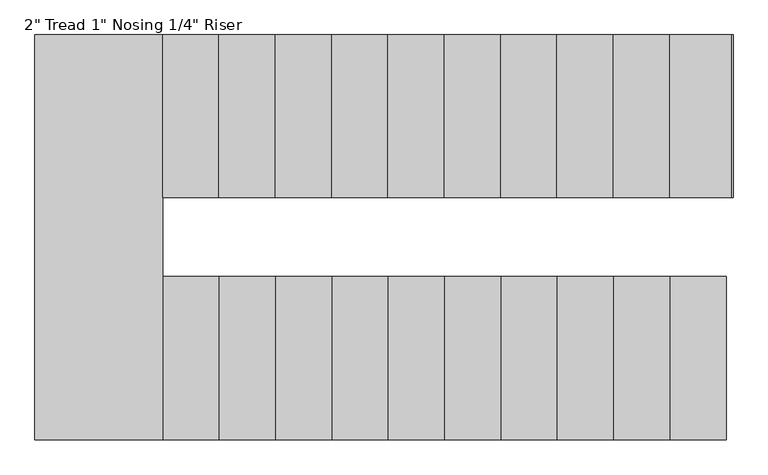
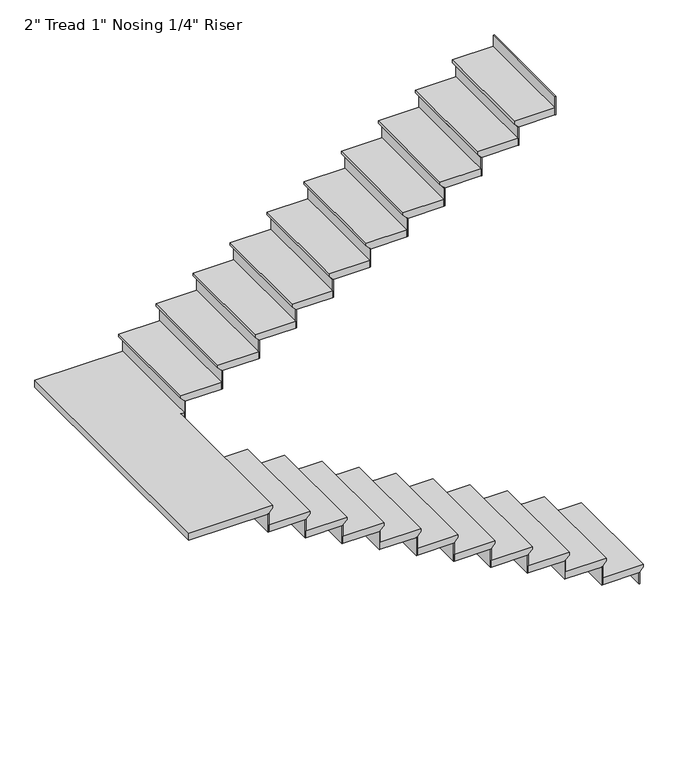
"""IFC4 building model written with IfcOpenShell, lengths in millimetres: stair flight geometry."""

from ifc_helpers import new_model, si_unit, origin, place, context, project, spatial, faceted_brep, source, transform, mapped, element, save


def stair_flight_e10cbaa8(model_context):
    return source(origin(), model_context, "Body", "Brep", [
        faceted_brep([(-3117.2664982, -6914.3822004, 6513.3681818), (-3117.2664982, -6914.3822004, 6532.4181818), (-3117.2664982, -7650.9822004, 6532.4181818), (-3117.2664982, -7650.9822004, 6513.3681818), (-3142.6664982, -6914.3822004, 6487.9681818), (-3142.6664982, -7650.9822004, 6487.9681818), (-3396.6664982, -6914.3822004, 6532.4181818), (-3396.6664982, -7650.9822004, 6532.4181818), (-3142.6664982, -7650.9822004, 6481.6181818), (-3396.6664982, -7650.9822004, 6481.6181818), (-3396.6664982, -6914.3822004, 6481.6181818), (-3142.6664982, -6914.3822004, 6481.6181818)], [[[0, 1, 2, 3]], [[4, 0, 3, 5]], [[2, 1, 6, 7]], [[8, 9, 10, 11]], [[2, 7, 9, 8, 5, 3]], [[8, 11, 4, 5]], [[6, 1, 0, 4, 11, 10]], [[7, 6, 10, 9]]]),
        faceted_brep([(-3142.6664982, -6914.3822004, 6481.6181818), (-3142.6664982, -6914.3822004, 6400.8), (-3149.0164982, -6914.3822004, 6400.8), (-3149.0164982, -6914.3822004, 6481.6181818), (-3142.6664982, -7650.9822004, 6481.6181818), (-3149.0164982, -7650.9822004, 6481.6181818), (-3149.0164982, -7650.9822004, 6400.8), (-3142.6664982, -7650.9822004, 6400.8)], [[[0, 1, 2, 3]], [[4, 5, 6, 7]], [[1, 0, 4, 7]], [[2, 1, 7, 6]], [[3, 2, 6, 5]], [[0, 3, 5, 4]]]),
        faceted_brep([(-3396.6664982, -6914.3822004, 6613.2363636), (-3396.6664982, -6914.3822004, 6481.6181818), (-3403.0164982, -6914.3822004, 6481.6181818), (-3403.0164982, -6914.3822004, 6613.2363636), (-3396.6664982, -7650.9822004, 6613.2363636), (-3403.0164982, -7650.9822004, 6613.2363636), (-3403.0164982, -7650.9822004, 6481.6181818), (-3396.6664982, -7650.9822004, 6481.6181818)], [[[0, 1, 2, 3]], [[4, 5, 6, 7]], [[1, 0, 4, 7]], [[2, 1, 7, 6]], [[3, 2, 6, 5]], [[0, 3, 5, 4]]]),
        faceted_brep([(-3371.2664982, -7650.9822004, 6664.0363636), (-3371.2664982, -6914.3822004, 6664.0363636), (-3650.6664982, -6914.3822004, 6664.0363636), (-3650.6664982, -7650.9822004, 6664.0363636), (-3396.6664982, -7650.9822004, 6613.2363636), (-3650.6664982, -7650.9822004, 6613.2363636), (-3650.6664982, -6914.3822004, 6613.2363636), (-3396.6664982, -6914.3822004, 6613.2363636), (-3396.6664982, -7650.9822004, 6619.5863636), (-3371.2664982, -7650.9822004, 6644.9863636), (-3396.6664982, -6914.3822004, 6619.5863636), (-3371.2664982, -6914.3822004, 6644.9863636)], [[[0, 1, 2, 3]], [[4, 5, 6, 7]], [[0, 3, 5, 4, 8, 9]], [[4, 7, 10, 8]], [[2, 1, 11, 10, 7, 6]], [[3, 2, 6, 5]], [[11, 1, 0, 9]], [[10, 11, 9, 8]]]),
        faceted_brep([(-3650.6664982, -6914.3822004, 6744.8545455), (-3650.6664982, -6914.3822004, 6613.2363636), (-3657.0164982, -6914.3822004, 6613.2363636), (-3657.0164982, -6914.3822004, 6744.8545455), (-3650.6664982, -7650.9822004, 6744.8545455), (-3657.0164982, -7650.9822004, 6744.8545455), (-3657.0164982, -7650.9822004, 6613.2363636), (-3650.6664982, -7650.9822004, 6613.2363636)], [[[0, 1, 2, 3]], [[4, 5, 6, 7]], [[1, 0, 4, 7]], [[2, 1, 7, 6]], [[3, 2, 6, 5]], [[0, 3, 5, 4]]]),
        faceted_brep([(-3625.2664982, -7650.9822004, 6795.6545455), (-3625.2664982, -6914.3822004, 6795.6545455), (-3904.6664982, -6914.3822004, 6795.6545455), (-3904.6664982, -7650.9822004, 6795.6545455), (-3650.6664982, -7650.9822004, 6744.8545455), (-3904.6664982, -7650.9822004, 6744.8545455), (-3904.6664982, -6914.3822004, 6744.8545455), (-3650.6664982, -6914.3822004, 6744.8545455), (-3650.6664982, -7650.9822004, 6751.2045455), (-3625.2664982, -7650.9822004, 6776.6045455), (-3650.6664982, -6914.3822004, 6751.2045455), (-3625.2664982, -6914.3822004, 6776.6045455)], [[[0, 1, 2, 3]], [[4, 5, 6, 7]], [[0, 3, 5, 4, 8, 9]], [[4, 7, 10, 8]], [[2, 1, 11, 10, 7, 6]], [[3, 2, 6, 5]], [[11, 1, 0, 9]], [[10, 11, 9, 8]]]),
        faceted_brep([(-3904.6664982, -6914.3822004, 6876.4727273), (-3904.6664982, -6914.3822004, 6744.8545455), (-3911.0164982, -6914.3822004, 6744.8545455), (-3911.0164982, -6914.3822004, 6876.4727273), (-3904.6664982, -7650.9822004, 6876.4727273), (-3911.0164982, -7650.9822004, 6876.4727273), (-3911.0164982, -7650.9822004, 6744.8545455), (-3904.6664982, -7650.9822004, 6744.8545455)], [[[0, 1, 2, 3]], [[4, 5, 6, 7]], [[1, 0, 4, 7]], [[2, 1, 7, 6]], [[3, 2, 6, 5]], [[0, 3, 5, 4]]]),
        faceted_brep([(-3879.2664982, -7650.9822004, 6927.2727273), (-3879.2664982, -6914.3822004, 6927.2727273), (-4158.6664982, -6914.3822004, 6927.2727273), (-4158.6664982, -7650.9822004, 6927.2727273), (-3904.6664982, -7650.9822004, 6876.4727273), (-4158.6664982, -7650.9822004, 6876.4727273), (-4158.6664982, -6914.3822004, 6876.4727273), (-3904.6664982, -6914.3822004, 6876.4727273), (-3904.6664982, -7650.9822004, 6882.8227273), (-3879.2664982, -7650.9822004, 6908.2227273), (-3904.6664982, -6914.3822004, 6882.8227273), (-3879.2664982, -6914.3822004, 6908.2227273)], [[[0, 1, 2, 3]], [[4, 5, 6, 7]], [[0, 3, 5, 4, 8, 9]], [[4, 7, 10, 8]], [[2, 1, 11, 10, 7, 6]], [[3, 2, 6, 5]], [[11, 1, 0, 9]], [[10, 11, 9, 8]]]),
        faceted_brep([(-4158.6664982, -6914.3822004, 7008.0909091), (-4158.6664982, -6914.3822004, 6876.4727273), (-4165.0164982, -6914.3822004, 6876.4727273), (-4165.0164982, -6914.3822004, 7008.0909091), (-4158.6664982, -7650.9822004, 7008.0909091), (-4165.0164982, -7650.9822004, 7008.0909091), (-4165.0164982, -7650.9822004, 6876.4727273), (-4158.6664982, -7650.9822004, 6876.4727273)], [[[0, 1, 2, 3]], [[4, 5, 6, 7]], [[1, 0, 4, 7]], [[2, 1, 7, 6]], [[3, 2, 6, 5]], [[0, 3, 5, 4]]]),
        faceted_brep([(-4133.2664982, -7650.9822004, 7058.8909091), (-4133.2664982, -6914.3822004, 7058.8909091), (-4412.6664982, -6914.3822004, 7058.8909091), (-4412.6664982, -7650.9822004, 7058.8909091), (-4158.6664982, -7650.9822004, 7008.0909091), (-4412.6664982, -7650.9822004, 7008.0909091), (-4412.6664982, -6914.3822004, 7008.0909091), (-4158.6664982, -6914.3822004, 7008.0909091), (-4158.6664982, -7650.9822004, 7014.4409091), (-4133.2664982, -7650.9822004, 7039.8409091), (-4158.6664982, -6914.3822004, 7014.4409091), (-4133.2664982, -6914.3822004, 7039.8409091)], [[[0, 1, 2, 3]], [[4, 5, 6, 7]], [[0, 3, 5, 4, 8, 9]], [[4, 7, 10, 8]], [[2, 1, 11, 10, 7, 6]], [[3, 2, 6, 5]], [[11, 1, 0, 9]], [[10, 11, 9, 8]]]),
        faceted_brep([(-4412.6664982, -6914.3822004, 7139.7090909), (-4412.6664982, -6914.3822004, 7008.0909091), (-4419.0164982, -6914.3822004, 7008.0909091), (-4419.0164982, -6914.3822004, 7139.7090909), (-4412.6664982, -7650.9822004, 7139.7090909), (-4419.0164982, -7650.9822004, 7139.7090909), (-4419.0164982, -7650.9822004, 7008.0909091), (-4412.6664982, -7650.9822004, 7008.0909091)], [[[0, 1, 2, 3]], [[4, 5, 6, 7]], [[1, 0, 4, 7]], [[2, 1, 7, 6]], [[3, 2, 6, 5]], [[0, 3, 5, 4]]]),
        faceted_brep([(-4387.2664982, -7650.9822004, 7190.5090909), (-4387.2664982, -6914.3822004, 7190.5090909), (-4666.6664982, -6914.3822004, 7190.5090909), (-4666.6664982, -7650.9822004, 7190.5090909), (-4412.6664982, -7650.9822004, 7139.7090909), (-4666.6664982, -7650.9822004, 7139.7090909), (-4666.6664982, -6914.3822004, 7139.7090909), (-4412.6664982, -6914.3822004, 7139.7090909), (-4412.6664982, -7650.9822004, 7146.0590909), (-4387.2664982, -7650.9822004, 7171.4590909), (-4412.6664982, -6914.3822004, 7146.0590909), (-4387.2664982, -6914.3822004, 7171.4590909)], [[[0, 1, 2, 3]], [[4, 5, 6, 7]], [[0, 3, 5, 4, 8, 9]], [[4, 7, 10, 8]], [[2, 1, 11, 10, 7, 6]], [[3, 2, 6, 5]], [[11, 1, 0, 9]], [[10, 11, 9, 8]]]),
        faceted_brep([(-4666.6664982, -6914.3822004, 7271.3272727), (-4666.6664982, -6914.3822004, 7139.7090909), (-4673.0164982, -6914.3822004, 7139.7090909), (-4673.0164982, -6914.3822004, 7271.3272727), (-4666.6664982, -7650.9822004, 7271.3272727), (-4673.0164982, -7650.9822004, 7271.3272727), (-4673.0164982, -7650.9822004, 7139.7090909), (-4666.6664982, -7650.9822004, 7139.7090909)], [[[0, 1, 2, 3]], [[4, 5, 6, 7]], [[1, 0, 4, 7]], [[2, 1, 7, 6]], [[3, 2, 6, 5]], [[0, 3, 5, 4]]]),
        faceted_brep([(-4641.2664982, -7650.9822004, 7322.1272727), (-4641.2664982, -6914.3822004, 7322.1272727), (-4920.6664982, -6914.3822004, 7322.1272727), (-4920.6664982, -7650.9822004, 7322.1272727), (-4666.6664982, -7650.9822004, 7271.3272727), (-4920.6664982, -7650.9822004, 7271.3272727), (-4920.6664982, -6914.3822004, 7271.3272727), (-4666.6664982, -6914.3822004, 7271.3272727), (-4666.6664982, -7650.9822004, 7277.6772727), (-4641.2664982, -7650.9822004, 7303.0772727), (-4666.6664982, -6914.3822004, 7277.6772727), (-4641.2664982, -6914.3822004, 7303.0772727)], [[[0, 1, 2, 3]], [[4, 5, 6, 7]], [[0, 3, 5, 4, 8, 9]], [[4, 7, 10, 8]], [[2, 1, 11, 10, 7, 6]], [[3, 2, 6, 5]], [[11, 1, 0, 9]], [[10, 11, 9, 8]]]),
        faceted_brep([(-4920.6664982, -6914.3822004, 7402.9454545), (-4920.6664982, -6914.3822004, 7271.3272727), (-4927.0164982, -6914.3822004, 7271.3272727), (-4927.0164982, -6914.3822004, 7402.9454545), (-4920.6664982, -7650.9822004, 7402.9454545), (-4927.0164982, -7650.9822004, 7402.9454545), (-4927.0164982, -7650.9822004, 7271.3272727), (-4920.6664982, -7650.9822004, 7271.3272727)], [[[0, 1, 2, 3]], [[4, 5, 6, 7]], [[1, 0, 4, 7]], [[2, 1, 7, 6]], [[3, 2, 6, 5]], [[0, 3, 5, 4]]]),
        faceted_brep([(-4895.2664982, -7650.9822004, 7453.7454545), (-4895.2664982, -6914.3822004, 7453.7454545), (-5174.6664982, -6914.3822004, 7453.7454545), (-5174.6664982, -7650.9822004, 7453.7454545), (-4920.6664982, -7650.9822004, 7402.9454545), (-5174.6664982, -7650.9822004, 7402.9454545), (-5174.6664982, -6914.3822004, 7402.9454545), (-4920.6664982, -6914.3822004, 7402.9454545), (-4920.6664982, -7650.9822004, 7409.2954545), (-4895.2664982, -7650.9822004, 7434.6954545), (-4920.6664982, -6914.3822004, 7409.2954545), (-4895.2664982, -6914.3822004, 7434.6954545)], [[[0, 1, 2, 3]], [[4, 5, 6, 7]], [[0, 3, 5, 4, 8, 9]], [[4, 7, 10, 8]], [[2, 1, 11, 10, 7, 6]], [[3, 2, 6, 5]], [[11, 1, 0, 9]], [[10, 11, 9, 8]]]),
        faceted_brep([(-5174.6664982, -6914.3822004, 7534.5636364), (-5174.6664982, -6914.3822004, 7402.9454545), (-5181.0164982, -6914.3822004, 7402.9454545), (-5181.0164982, -6914.3822004, 7534.5636364), (-5174.6664982, -7650.9822004, 7534.5636364), (-5181.0164982, -7650.9822004, 7534.5636364), (-5181.0164982, -7650.9822004, 7402.9454545), (-5174.6664982, -7650.9822004, 7402.9454545)], [[[0, 1, 2, 3]], [[4, 5, 6, 7]], [[1, 0, 4, 7]], [[2, 1, 7, 6]], [[3, 2, 6, 5]], [[0, 3, 5, 4]]]),
        faceted_brep([(-5149.2664982, -7650.9822004, 7585.3636364), (-5149.2664982, -6914.3822004, 7585.3636364), (-5428.6664982, -6914.3822004, 7585.3636364), (-5428.6664982, -7650.9822004, 7585.3636364), (-5174.6664982, -7650.9822004, 7534.5636364), (-5428.6664982, -7650.9822004, 7534.5636364), (-5428.6664982, -6914.3822004, 7534.5636364), (-5174.6664982, -6914.3822004, 7534.5636364), (-5174.6664982, -7650.9822004, 7540.9136364), (-5149.2664982, -7650.9822004, 7566.3136364), (-5174.6664982, -6914.3822004, 7540.9136364), (-5149.2664982, -6914.3822004, 7566.3136364)], [[[0, 1, 2, 3]], [[4, 5, 6, 7]], [[0, 3, 5, 4, 8, 9]], [[4, 7, 10, 8]], [[2, 1, 11, 10, 7, 6]], [[3, 2, 6, 5]], [[11, 1, 0, 9]], [[10, 11, 9, 8]]]),
        faceted_brep([(-5428.6664982, -6914.3822004, 7666.1818182), (-5428.6664982, -6914.3822004, 7534.5636364), (-5435.0164982, -6914.3822004, 7534.5636364), (-5435.0164982, -6914.3822004, 7666.1818182), (-5428.6664982, -7650.9822004, 7666.1818182), (-5435.0164982, -7650.9822004, 7666.1818182), (-5435.0164982, -7650.9822004, 7534.5636364), (-5428.6664982, -7650.9822004, 7534.5636364)], [[[0, 1, 2, 3]], [[4, 5, 6, 7]], [[1, 0, 4, 7]], [[2, 1, 7, 6]], [[3, 2, 6, 5]], [[0, 3, 5, 4]]]),
        faceted_brep([(-5403.2664982, -7650.9822004, 7716.9818182), (-5403.2664982, -6914.3822004, 7716.9818182), (-5682.6664982, -6914.3822004, 7716.9818182), (-5682.6664982, -7650.9822004, 7716.9818182), (-5428.6664982, -7650.9822004, 7666.1818182), (-5682.6664982, -7650.9822004, 7666.1818182), (-5682.6664982, -6914.3822004, 7666.1818182), (-5428.6664982, -6914.3822004, 7666.1818182), (-5428.6664982, -7650.9822004, 7672.5318182), (-5403.2664982, -7650.9822004, 7697.9318182), (-5428.6664982, -6914.3822004, 7672.5318182), (-5403.2664982, -6914.3822004, 7697.9318182)], [[[0, 1, 2, 3]], [[4, 5, 6, 7]], [[0, 3, 5, 4, 8, 9]], [[4, 7, 10, 8]], [[2, 1, 11, 10, 7, 6]], [[3, 2, 6, 5]], [[11, 1, 0, 9]], [[10, 11, 9, 8]]]),
        faceted_brep([(-5682.6664982, -6914.3822004, 7797.8), (-5682.6664982, -6914.3822004, 7666.1818182), (-5689.0164982, -6914.3822004, 7666.1818182), (-5689.0164982, -6914.3822004, 7797.8), (-5682.6664982, -7650.9822004, 7797.8), (-5689.0164982, -7650.9822004, 7797.8), (-5689.0164982, -7650.9822004, 7666.1818182), (-5682.6664982, -7650.9822004, 7666.1818182)], [[[0, 1, 2, 3]], [[4, 5, 6, 7]], [[1, 0, 4, 7]], [[2, 1, 7, 6]], [[3, 2, 6, 5]], [[0, 3, 5, 4]]]),
        faceted_brep([(-5631.8664982, -5824.7082131, 7848.6), (-6232.5131972, -5824.7082131, 7848.6), (-6232.5131972, -7650.9822004, 7848.6), (-5657.2664982, -7650.9822004, 7848.6), (-5657.2664982, -6558.7822004, 7848.6), (-5631.8664982, -6558.7822004, 7848.6), (-6232.5131972, -5824.7082131, 7797.8), (-5631.8664982, -5824.7082131, 7797.8), (-5631.8664982, -6558.7822004, 7797.8), (-5657.2664982, -6558.7822004, 7797.8), (-5657.2664982, -6914.3822004, 7797.8), (-5682.6664982, -6914.3822004, 7797.8), (-5682.6664982, -7650.9822004, 7797.8), (-6232.5131972, -7650.9822004, 7797.8), (-5682.6664982, -6914.3822004, 7804.15), (-5682.6664982, -7650.9822004, 7804.15), (-5657.2664982, -7650.9822004, 7829.55), (-5657.2664982, -6914.3822004, 7829.55)], [[[0, 1, 2, 3, 4, 5]], [[6, 7, 8, 9, 10, 11, 12, 13]], [[1, 0, 7, 6]], [[2, 1, 6, 13]], [[12, 11, 14, 15]], [[4, 3, 16, 17, 10, 9]], [[5, 4, 9, 8]], [[0, 5, 8, 7]], [[16, 15, 14, 17]], [[3, 2, 13, 12, 15, 16]], [[11, 10, 17, 14]]]),
        faceted_brep([(-5631.8664982, -6558.7822004, 7929.4181818), (-5631.8664982, -6558.7822004, 7797.8), (-5625.5164982, -6558.7822004, 7797.8), (-5625.5164982, -6558.7822004, 7929.4181818), (-5631.8664982, -5824.7082131, 7929.4181818), (-5625.5164982, -5824.7082131, 7929.4181818), (-5625.5164982, -5824.7082131, 7797.8), (-5631.8664982, -5824.7082131, 7797.8)], [[[0, 1, 2, 3]], [[4, 5, 6, 7]], [[1, 0, 4, 7]], [[2, 1, 7, 6]], [[3, 2, 6, 5]], [[0, 3, 5, 4]]]),
        faceted_brep([(-5657.2664982, -5824.7082131, 7980.2181818), (-5657.2664982, -6558.7822004, 7980.2181818), (-5377.8664982, -6558.7822004, 7980.2181818), (-5377.8664982, -5824.7082131, 7980.2181818), (-5631.8664982, -5824.7082131, 7929.4181818), (-5377.8664982, -5824.7082131, 7929.4181818), (-5377.8664982, -6558.7822004, 7929.4181818), (-5631.8664982, -6558.7822004, 7929.4181818), (-5631.8664982, -5824.7082131, 7935.7681818), (-5657.2664982, -5824.7082131, 7961.1681818), (-5631.8664982, -6558.7822004, 7935.7681818), (-5657.2664982, -6558.7822004, 7961.1681818)], [[[0, 1, 2, 3]], [[4, 5, 6, 7]], [[0, 3, 5, 4, 8, 9]], [[4, 7, 10, 8]], [[2, 1, 11, 10, 7, 6]], [[3, 2, 6, 5]], [[11, 1, 0, 9]], [[10, 11, 9, 8]]]),
        faceted_brep([(-5377.8664982, -6558.7822004, 8061.0363636), (-5377.8664982, -6558.7822004, 7929.4181818), (-5371.5164982, -6558.7822004, 7929.4181818), (-5371.5164982, -6558.7822004, 8061.0363636), (-5377.8664982, -5824.7082131, 8061.0363636), (-5371.5164982, -5824.7082131, 8061.0363636), (-5371.5164982, -5824.7082131, 7929.4181818), (-5377.8664982, -5824.7082131, 7929.4181818)], [[[0, 1, 2, 3]], [[4, 5, 6, 7]], [[1, 0, 4, 7]], [[2, 1, 7, 6]], [[3, 2, 6, 5]], [[0, 3, 5, 4]]]),
        faceted_brep([(-5403.2664982, -5824.7082131, 8111.8363636), (-5403.2664982, -6558.7822004, 8111.8363636), (-5123.8664982, -6558.7822004, 8111.8363636), (-5123.8664982, -5824.7082131, 8111.8363636), (-5377.8664982, -5824.7082131, 8061.0363636), (-5123.8664982, -5824.7082131, 8061.0363636), (-5123.8664982, -6558.7822004, 8061.0363636), (-5377.8664982, -6558.7822004, 8061.0363636), (-5377.8664982, -5824.7082131, 8067.3863636), (-5403.2664982, -5824.7082131, 8092.7863636), (-5377.8664982, -6558.7822004, 8067.3863636), (-5403.2664982, -6558.7822004, 8092.7863636)], [[[0, 1, 2, 3]], [[4, 5, 6, 7]], [[0, 3, 5, 4, 8, 9]], [[4, 7, 10, 8]], [[2, 1, 11, 10, 7, 6]], [[3, 2, 6, 5]], [[11, 1, 0, 9]], [[10, 11, 9, 8]]]),
        faceted_brep([(-5123.8664982, -6558.7822004, 8192.6545455), (-5123.8664982, -6558.7822004, 8061.0363636), (-5117.5164982, -6558.7822004, 8061.0363636), (-5117.5164982, -6558.7822004, 8192.6545455), (-5123.8664982, -5824.7082131, 8192.6545455), (-5117.5164982, -5824.7082131, 8192.6545455), (-5117.5164982, -5824.7082131, 8061.0363636), (-5123.8664982, -5824.7082131, 8061.0363636)], [[[0, 1, 2, 3]], [[4, 5, 6, 7]], [[1, 0, 4, 7]], [[2, 1, 7, 6]], [[3, 2, 6, 5]], [[0, 3, 5, 4]]]),
        faceted_brep([(-5149.2664982, -5824.7082131, 8243.4545455), (-5149.2664982, -6558.7822004, 8243.4545455), (-4869.8664982, -6558.7822004, 8243.4545455), (-4869.8664982, -5824.7082131, 8243.4545455), (-5123.8664982, -5824.7082131, 8192.6545455), (-4869.8664982, -5824.7082131, 8192.6545455), (-4869.8664982, -6558.7822004, 8192.6545455), (-5123.8664982, -6558.7822004, 8192.6545455), (-5123.8664982, -5824.7082131, 8199.0045455), (-5149.2664982, -5824.7082131, 8224.4045455), (-5123.8664982, -6558.7822004, 8199.0045455), (-5149.2664982, -6558.7822004, 8224.4045455)], [[[0, 1, 2, 3]], [[4, 5, 6, 7]], [[0, 3, 5, 4, 8, 9]], [[4, 7, 10, 8]], [[2, 1, 11, 10, 7, 6]], [[3, 2, 6, 5]], [[11, 1, 0, 9]], [[10, 11, 9, 8]]]),
        faceted_brep([(-4869.8664982, -6558.7822004, 8324.2727273), (-4869.8664982, -6558.7822004, 8192.6545455), (-4863.5164982, -6558.7822004, 8192.6545455), (-4863.5164982, -6558.7822004, 8324.2727273), (-4869.8664982, -5824.7082131, 8324.2727273), (-4863.5164982, -5824.7082131, 8324.2727273), (-4863.5164982, -5824.7082131, 8192.6545455), (-4869.8664982, -5824.7082131, 8192.6545455)], [[[0, 1, 2, 3]], [[4, 5, 6, 7]], [[1, 0, 4, 7]], [[2, 1, 7, 6]], [[3, 2, 6, 5]], [[0, 3, 5, 4]]]),
        faceted_brep([(-4895.2664982, -5824.7082131, 8375.0727273), (-4895.2664982, -6558.7822004, 8375.0727273), (-4615.8664982, -6558.7822004, 8375.0727273), (-4615.8664982, -5824.7082131, 8375.0727273), (-4869.8664982, -5824.7082131, 8324.2727273), (-4615.8664982, -5824.7082131, 8324.2727273), (-4615.8664982, -6558.7822004, 8324.2727273), (-4869.8664982, -6558.7822004, 8324.2727273), (-4869.8664982, -5824.7082131, 8330.6227273), (-4895.2664982, -5824.7082131, 8356.0227273), (-4869.8664982, -6558.7822004, 8330.6227273), (-4895.2664982, -6558.7822004, 8356.0227273)], [[[0, 1, 2, 3]], [[4, 5, 6, 7]], [[0, 3, 5, 4, 8, 9]], [[4, 7, 10, 8]], [[2, 1, 11, 10, 7, 6]], [[3, 2, 6, 5]], [[11, 1, 0, 9]], [[10, 11, 9, 8]]]),
        faceted_brep([(-4615.8664982, -6558.7822004, 8455.8909091), (-4615.8664982, -6558.7822004, 8324.2727273), (-4609.5164982, -6558.7822004, 8324.2727273), (-4609.5164982, -6558.7822004, 8455.8909091), (-4615.8664982, -5824.7082131, 8455.8909091), (-4609.5164982, -5824.7082131, 8455.8909091), (-4609.5164982, -5824.7082131, 8324.2727273), (-4615.8664982, -5824.7082131, 8324.2727273)], [[[0, 1, 2, 3]], [[4, 5, 6, 7]], [[1, 0, 4, 7]], [[2, 1, 7, 6]], [[3, 2, 6, 5]], [[0, 3, 5, 4]]]),
        faceted_brep([(-4641.2664982, -5824.7082131, 8506.6909091), (-4641.2664982, -6558.7822004, 8506.6909091), (-4361.8664982, -6558.7822004, 8506.6909091), (-4361.8664982, -5824.7082131, 8506.6909091), (-4615.8664982, -5824.7082131, 8455.8909091), (-4361.8664982, -5824.7082131, 8455.8909091), (-4361.8664982, -6558.7822004, 8455.8909091), (-4615.8664982, -6558.7822004, 8455.8909091), (-4615.8664982, -5824.7082131, 8462.2409091), (-4641.2664982, -5824.7082131, 8487.6409091), (-4615.8664982, -6558.7822004, 8462.2409091), (-4641.2664982, -6558.7822004, 8487.6409091)], [[[0, 1, 2, 3]], [[4, 5, 6, 7]], [[0, 3, 5, 4, 8, 9]], [[4, 7, 10, 8]], [[2, 1, 11, 10, 7, 6]], [[3, 2, 6, 5]], [[11, 1, 0, 9]], [[10, 11, 9, 8]]]),
        faceted_brep([(-4361.8664982, -6558.7822004, 8587.5090909), (-4361.8664982, -6558.7822004, 8455.8909091), (-4355.5164982, -6558.7822004, 8455.8909091), (-4355.5164982, -6558.7822004, 8587.5090909), (-4361.8664982, -5824.7082131, 8587.5090909), (-4355.5164982, -5824.7082131, 8587.5090909), (-4355.5164982, -5824.7082131, 8455.8909091), (-4361.8664982, -5824.7082131, 8455.8909091)], [[[0, 1, 2, 3]], [[4, 5, 6, 7]], [[1, 0, 4, 7]], [[2, 1, 7, 6]], [[3, 2, 6, 5]], [[0, 3, 5, 4]]]),
        faceted_brep([(-4387.2664982, -5824.7082131, 8638.3090909), (-4387.2664982, -6558.7822004, 8638.3090909), (-4107.8664982, -6558.7822004, 8638.3090909), (-4107.8664982, -5824.7082131, 8638.3090909), (-4361.8664982, -5824.7082131, 8587.5090909), (-4107.8664982, -5824.7082131, 8587.5090909), (-4107.8664982, -6558.7822004, 8587.5090909), (-4361.8664982, -6558.7822004, 8587.5090909), (-4361.8664982, -5824.7082131, 8593.8590909), (-4387.2664982, -5824.7082131, 8619.2590909), (-4361.8664982, -6558.7822004, 8593.8590909), (-4387.2664982, -6558.7822004, 8619.2590909)], [[[0, 1, 2, 3]], [[4, 5, 6, 7]], [[0, 3, 5, 4, 8, 9]], [[4, 7, 10, 8]], [[2, 1, 11, 10, 7, 6]], [[3, 2, 6, 5]], [[11, 1, 0, 9]], [[10, 11, 9, 8]]]),
        faceted_brep([(-4107.8664982, -6558.7822004, 8719.1272727), (-4107.8664982, -6558.7822004, 8587.5090909), (-4101.5164982, -6558.7822004, 8587.5090909), (-4101.5164982, -6558.7822004, 8719.1272727), (-4107.8664982, -5824.7082131, 8719.1272727), (-4101.5164982, -5824.7082131, 8719.1272727), (-4101.5164982, -5824.7082131, 8587.5090909), (-4107.8664982, -5824.7082131, 8587.5090909)], [[[0, 1, 2, 3]], [[4, 5, 6, 7]], [[1, 0, 4, 7]], [[2, 1, 7, 6]], [[3, 2, 6, 5]], [[0, 3, 5, 4]]]),
        faceted_brep([(-4133.2664982, -5824.7082131, 8769.9272727), (-4133.2664982, -6558.7822004, 8769.9272727), (-3853.8664982, -6558.7822004, 8769.9272727), (-3853.8664982, -5824.7082131, 8769.9272727), (-4107.8664982, -5824.7082131, 8719.1272727), (-3853.8664982, -5824.7082131, 8719.1272727), (-3853.8664982, -6558.7822004, 8719.1272727), (-4107.8664982, -6558.7822004, 8719.1272727), (-4107.8664982, -5824.7082131, 8725.4772727), (-4133.2664982, -5824.7082131, 8750.8772727), (-4107.8664982, -6558.7822004, 8725.4772727), (-4133.2664982, -6558.7822004, 8750.8772727)], [[[0, 1, 2, 3]], [[4, 5, 6, 7]], [[0, 3, 5, 4, 8, 9]], [[4, 7, 10, 8]], [[2, 1, 11, 10, 7, 6]], [[3, 2, 6, 5]], [[11, 1, 0, 9]], [[10, 11, 9, 8]]]),
        faceted_brep([(-3853.8664982, -6558.7822004, 8850.7454545), (-3853.8664982, -6558.7822004, 8719.1272727), (-3847.5164982, -6558.7822004, 8719.1272727), (-3847.5164982, -6558.7822004, 8850.7454545), (-3853.8664982, -5824.7082131, 8850.7454545), (-3847.5164982, -5824.7082131, 8850.7454545), (-3847.5164982, -5824.7082131, 8719.1272727), (-3853.8664982, -5824.7082131, 8719.1272727)], [[[0, 1, 2, 3]], [[4, 5, 6, 7]], [[1, 0, 4, 7]], [[2, 1, 7, 6]], [[3, 2, 6, 5]], [[0, 3, 5, 4]]]),
        faceted_brep([(-3879.2664982, -5824.7082131, 8901.5454545), (-3879.2664982, -6558.7822004, 8901.5454545), (-3599.8664982, -6558.7822004, 8901.5454545), (-3599.8664982, -5824.7082131, 8901.5454545), (-3853.8664982, -5824.7082131, 8850.7454545), (-3599.8664982, -5824.7082131, 8850.7454545), (-3599.8664982, -6558.7822004, 8850.7454545), (-3853.8664982, -6558.7822004, 8850.7454545), (-3853.8664982, -5824.7082131, 8857.0954545), (-3879.2664982, -5824.7082131, 8882.4954545), (-3853.8664982, -6558.7822004, 8857.0954545), (-3879.2664982, -6558.7822004, 8882.4954545)], [[[0, 1, 2, 3]], [[4, 5, 6, 7]], [[0, 3, 5, 4, 8, 9]], [[4, 7, 10, 8]], [[2, 1, 11, 10, 7, 6]], [[3, 2, 6, 5]], [[11, 1, 0, 9]], [[10, 11, 9, 8]]]),
        faceted_brep([(-3599.8664982, -6558.7822004, 8982.3636364), (-3599.8664982, -6558.7822004, 8850.7454545), (-3593.5164982, -6558.7822004, 8850.7454545), (-3593.5164982, -6558.7822004, 8982.3636364), (-3599.8664982, -5824.7082131, 8982.3636364), (-3593.5164982, -5824.7082131, 8982.3636364), (-3593.5164982, -5824.7082131, 8850.7454545), (-3599.8664982, -5824.7082131, 8850.7454545)], [[[0, 1, 2, 3]], [[4, 5, 6, 7]], [[1, 0, 4, 7]], [[2, 1, 7, 6]], [[3, 2, 6, 5]], [[0, 3, 5, 4]]]),
        faceted_brep([(-3625.2664982, -5824.7082131, 9033.1636364), (-3625.2664982, -6558.7822004, 9033.1636364), (-3345.8664982, -6558.7822004, 9033.1636364), (-3345.8664982, -5824.7082131, 9033.1636364), (-3599.8664982, -5824.7082131, 8982.3636364), (-3345.8664982, -5824.7082131, 8982.3636364), (-3345.8664982, -6558.7822004, 8982.3636364), (-3599.8664982, -6558.7822004, 8982.3636364), (-3599.8664982, -5824.7082131, 8988.7136364), (-3625.2664982, -5824.7082131, 9014.1136364), (-3599.8664982, -6558.7822004, 8988.7136364), (-3625.2664982, -6558.7822004, 9014.1136364)], [[[0, 1, 2, 3]], [[4, 5, 6, 7]], [[0, 3, 5, 4, 8, 9]], [[4, 7, 10, 8]], [[2, 1, 11, 10, 7, 6]], [[3, 2, 6, 5]], [[11, 1, 0, 9]], [[10, 11, 9, 8]]]),
        faceted_brep([(-3345.8664982, -6558.7822004, 9113.9818182), (-3345.8664982, -6558.7822004, 8982.3636364), (-3339.5164982, -6558.7822004, 8982.3636364), (-3339.5164982, -6558.7822004, 9113.9818182), (-3345.8664982, -5824.7082131, 9113.9818182), (-3339.5164982, -5824.7082131, 9113.9818182), (-3339.5164982, -5824.7082131, 8982.3636364), (-3345.8664982, -5824.7082131, 8982.3636364)], [[[0, 1, 2, 3]], [[4, 5, 6, 7]], [[1, 0, 4, 7]], [[2, 1, 7, 6]], [[3, 2, 6, 5]], [[0, 3, 5, 4]]]),
        faceted_brep([(-3091.8664982, -6558.7822004, 9245.6), (-3091.8664982, -6558.7822004, 9113.9818182), (-3085.5164982, -6558.7822004, 9113.9818182), (-3085.5164982, -6558.7822004, 9245.6), (-3091.8664982, -5824.7082131, 9245.6), (-3085.5164982, -5824.7082131, 9245.6), (-3085.5164982, -5824.7082131, 9113.9818182), (-3091.8664982, -5824.7082131, 9113.9818182)], [[[0, 1, 2, 3]], [[4, 5, 6, 7]], [[1, 0, 4, 7]], [[2, 1, 7, 6]], [[3, 2, 6, 5]], [[0, 3, 5, 4]]]),
        faceted_brep([(-3371.2664982, -5824.7082131, 9164.7818182), (-3371.2664982, -6558.7822004, 9164.7818182), (-3091.8664982, -6558.7822004, 9164.7818182), (-3091.8664982, -5824.7082131, 9164.7818182), (-3345.8664982, -5824.7082131, 9113.9818182), (-3091.8664982, -5824.7082131, 9113.9818182), (-3091.8664982, -6558.7822004, 9113.9818182), (-3345.8664982, -6558.7822004, 9113.9818182), (-3345.8664982, -5824.7082131, 9120.3318182), (-3371.2664982, -5824.7082131, 9145.7318182), (-3345.8664982, -6558.7822004, 9120.3318182), (-3371.2664982, -6558.7822004, 9145.7318182)], [[[0, 1, 2, 3]], [[4, 5, 6, 7]], [[0, 3, 5, 4, 8, 9]], [[4, 7, 10, 8]], [[2, 1, 11, 10, 7, 6]], [[3, 2, 6, 5]], [[11, 1, 0, 9]], [[10, 11, 9, 8]]]),
    ])


if __name__ == "__main__":
    model = new_model("IFC4")
    model_context = context("Model", 3, world=origin())
    ifc_project = project(units=[si_unit("LENGTHUNIT", "METRE", prefix="MILLI")], contexts=[model_context])
    site = spatial("IfcSite", under=ifc_project)
    building = spatial("IfcBuilding", under=site)
    placement = place(None, origin())
    stair_flight_shape = stair_flight_e10cbaa8(model_context)
    element("IfcStairFlight", 1, ObjectType="2\" Tread 1\" Nosing 1/4\" Riser", at=placement, inside=building, context=model_context, shape_type="MappedRepresentation", body=[
        mapped(stair_flight_shape, transform((0.0, 0.0, 0.0), x_axis=(1.0, 0.0, 0.0), y_axis=(0.0, 1.0, 0.0), z_axis=(0.0, 0.0, 1.0))),
    ])
    save(model, "model.ifc")
